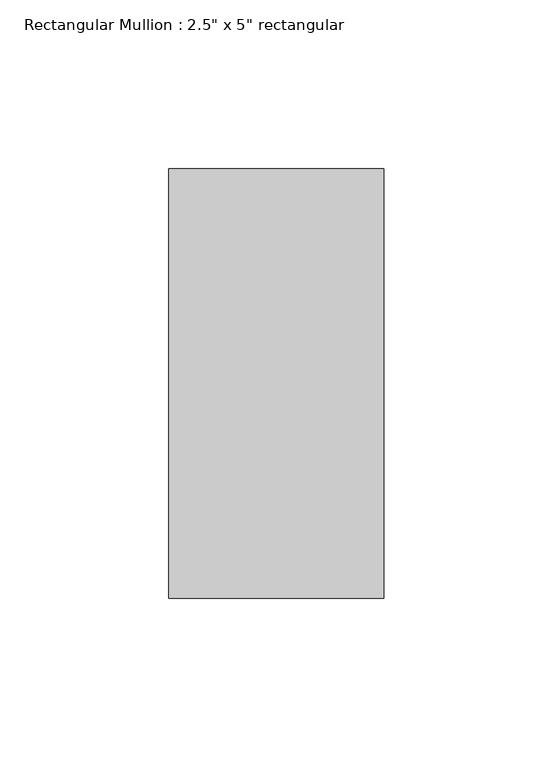
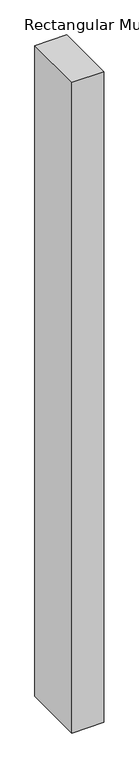
"""IFC4 building model written with IfcOpenShell, lengths in millimetres: member geometry."""

from ifc_helpers import new_model, si_unit, frame, origin, place, context, project, spatial, polyline, outline, extrude, source, transform, mapped, element, save


def member_a81ad59a(model_context):
    return source(origin(), model_context, "Body", "SweptSolid", [
        extrude(outline(polyline([(31.75, 63.5), (31.75, -63.5), (-31.75, -63.5), (-31.75, 63.5), (31.75, 63.5)])), frame((0.0, 0.0, -1365.4610041), z_axis=(0.0, 0.0, 1.0), x_axis=(1.0, 0.0, 0.0)), (0.0, 0.0, 1.0), 1365.4610041),
    ])


if __name__ == "__main__":
    model = new_model("IFC4")
    model_context = context("Model", 3, world=origin())
    ifc_project = project(units=[si_unit("LENGTHUNIT", "METRE", prefix="MILLI")], contexts=[model_context])
    site = spatial("IfcSite", under=ifc_project)
    building = spatial("IfcBuilding", under=site)
    placement = place(None, origin())
    member_shape = member_a81ad59a(model_context)
    element("IfcMember", 1, ObjectType="Rectangular Mullion : 2.5\" x 5\" rectangular", at=placement, inside=building, context=model_context, shape_type="MappedRepresentation", body=[
        mapped(member_shape, transform((0.0, 0.0, 0.0), x_axis=(1.0, 0.0, 0.0), y_axis=(0.0, 1.0, 0.0), z_axis=(0.0, 0.0, 1.0))),
    ])
    save(model, "model.ifc")

# Revit data of these elements
# Type "Rectangular Mullion : 2.5\" x 5\" rectangular"
#   built-in parameter 1007304 = 0.416667 (stored number, unit not read)
#   built-in parameter 1007301 = 0.104167 (stored number, unit not read)
#   built-in parameter 1007300 = 0.104167 (stored number, unit not read)
# Element 1 (IfcMember, "Rectangular Mullion : 2.5\" x 5\" rectangular")
#   Materials on its faces: "Aluminum"
# Materials
#   "Aluminum": class "Metal", colour RGB 247 247 247, transparency 0, Description = "Aluminum 6061", Cost = 0
